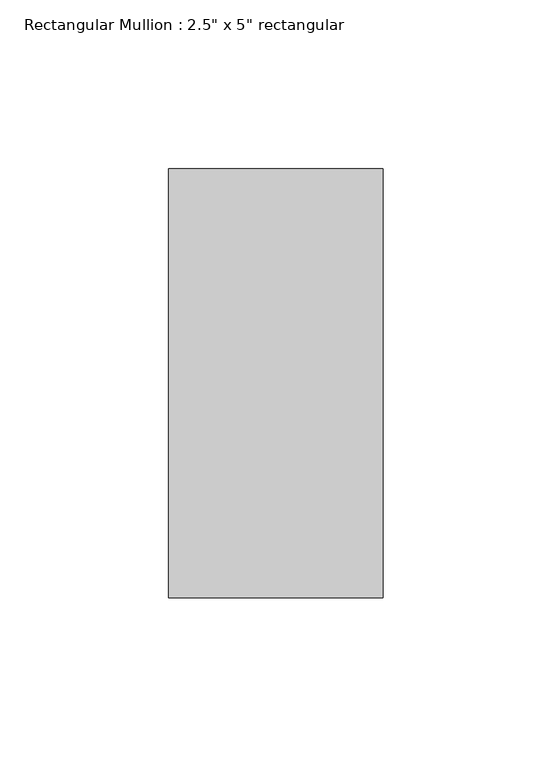
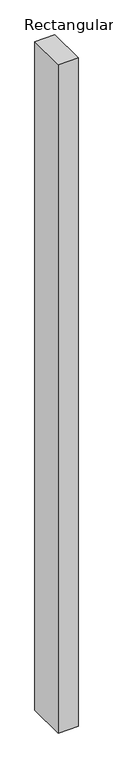
"""IFC4 building model written with IfcOpenShell, lengths in millimetres: member geometry."""

from ifc_helpers import new_model, si_unit, frame, origin, place, context, project, spatial, polyline, outline, extrude, source, transform, mapped, element, save


def member_88cd697c(model_context):
    return source(origin(), model_context, "Body", "SweptSolid", [
        extrude(outline(polyline([(31.75, 63.5), (31.75, -63.5), (-31.75, -63.5), (-31.75, 63.5), (31.75, 63.5)])), frame((0.0, 0.0, -2241.55), z_axis=(0.0, 0.0, 1.0), x_axis=(1.0, 0.0, 0.0)), (0.0, 0.0, 1.0), 2241.55),
    ])


if __name__ == "__main__":
    model = new_model("IFC4")
    model_context = context("Model", 3, world=origin())
    ifc_project = project(units=[si_unit("LENGTHUNIT", "METRE", prefix="MILLI")], contexts=[model_context])
    site = spatial("IfcSite", under=ifc_project)
    building = spatial("IfcBuilding", under=site)
    placement = place(None, origin())
    member_shape = member_88cd697c(model_context)
    element("IfcMember", 1, ObjectType="Rectangular Mullion : 2.5\" x 5\" rectangular", at=placement, inside=building, context=model_context, shape_type="MappedRepresentation", body=[
        mapped(member_shape, transform((0.0, 0.0, 0.0), x_axis=(1.0, 0.0, 0.0), y_axis=(0.0, 1.0, 0.0), z_axis=(0.0, 0.0, 1.0))),
    ])
    save(model, "model.ifc")

# Revit data of these elements
# Type "Rectangular Mullion : 2.5\" x 5\" rectangular"
#   built-in parameter 1007304 = 0.416667 (stored number, unit not read)
#   built-in parameter 1007301 = 0.104167 (stored number, unit not read)
#   built-in parameter 1007300 = 0.104167 (stored number, unit not read)
# Element 1 (IfcMember, "Rectangular Mullion : 2.5\" x 5\" rectangular")
#   Materials on its faces: "Aluminum"
# Materials
#   "Aluminum": class "Metal", colour RGB 247 247 247, transparency 0, Description = "Aluminum 6061", Cost = 0
